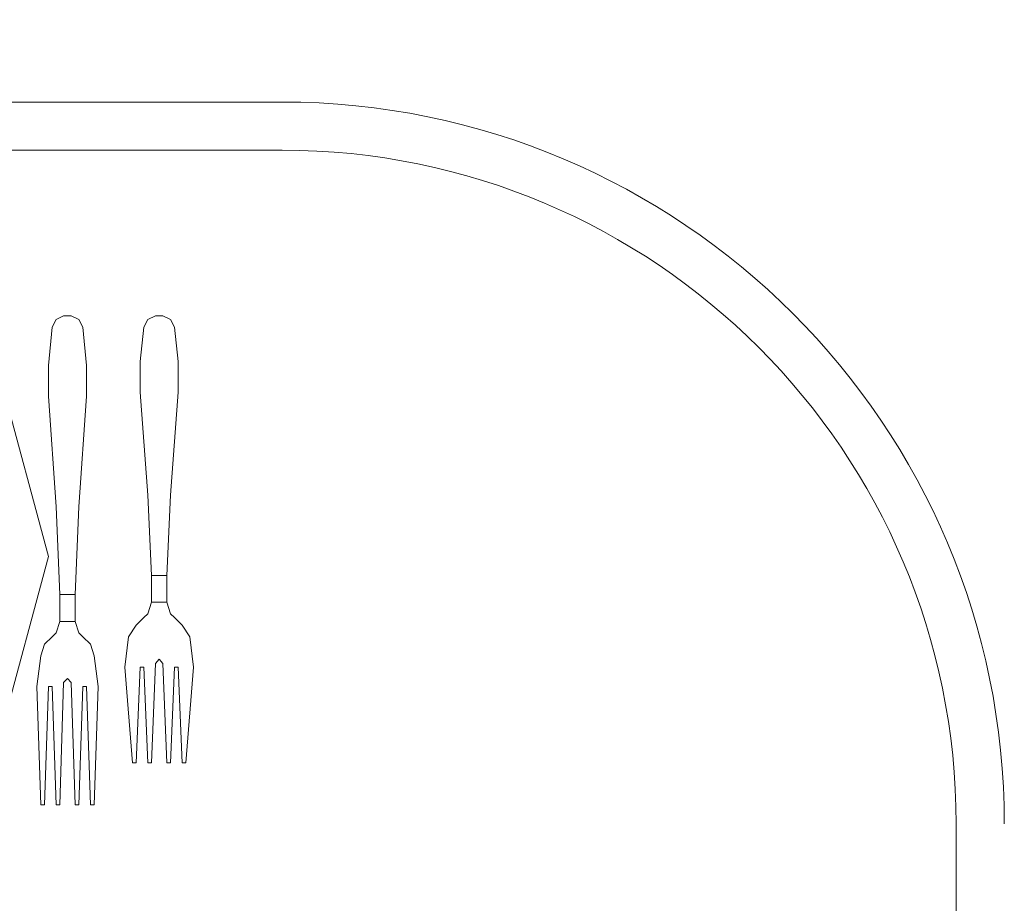
# Model space of a CAD drawing. Units: inches. Extents: x 375 to 1122, y 27 to 1069.
# Tile 64 of 155: x 731.16 to 747.02, y 311.59 to 325.82. Entities that reach past the tile are written whole.
import ezdxf

# ---------------------------------------------------------------- set-up
doc = ezdxf.new("R2010")
doc.units = ezdxf.units.IN
doc.layers.add('A-ANNO-DIMS', color=2, linetype='Continuous', lineweight=18)
doc.layers.add('Furniture', color=30, linetype='Continuous', lineweight=18)
doc.styles.get("Standard").update_dxf_attribs({"font": 'arial.ttf'})
doc.dimstyles.new('ISO-25', dxfattribs={"dimtxt": 12, "dimasz": 2.5, "dimexe": 1.5, "dimexo": 1.5, "dimtad": 1, "dimdec": 1, "dimlunit": 3, "dimtxsty": 'Standard', "dimblk": 'ARCHTICK', "dimcen": 2.5, "dimadec": 0, "dimazin": 0, "dimtfac": 1, "dimtdec": 1, "dimtmove": 0, "dimatfit": 3, "dimfxl": 1.5, "dimfxlon": 1, "dimarcsym": 0})

# ---------------------------------------------------------------- blocks, each defined once
blk = doc.blocks.new('A$C403C54AD')
for p, q in [((0.83575, 1.53256, -0.0006), (1.99923, 1.53256, -0.0006)), ((0.54488, 0.79569, -0.0006), (0.54488, 1.26108, -0.0006)), ((0.56427, 0.79569, -0.0006), (0.56427, 1.26108, -0.0006)), ((0.76029, 1.22386, -0.03201), (0.75567, 1.22078, -0.03155)), ((0.76029, 1.22386, -0.03509), (0.75567, 1.22078, -0.03463)), ((0.76798, 1.18538, -0.03201), (0.76336, 1.18384, -0.03155)), ((0.76798, 1.18538, -0.03509), (0.76336, 1.18384, -0.03463))]:
    blk.add_line(p, q)
for radius in [0.29087, 0.27148]:
    blk.add_arc((0.83575, 1.26108, -0.0006), radius, 90, 180)
for points, invisible_edges in [([(0.75567, 1.20231, -0.03155), (0.75567, 1.22078, -0.03155), (0.76029, 1.22386, -0.03201), (0.76029, 1.19923, -0.03201)], 5), ([(0.75567, 1.20231, -0.03463), (0.75567, 1.22078, -0.03463), (0.76029, 1.22386, -0.03509), (0.76029, 1.19923, -0.03509)], 5), ([(0.75567, 1.22078, -0.03155), (0.75567, 1.22078, -0.03463), (0.76029, 1.22386, -0.03509), (0.76029, 1.22386, -0.03201)], 4), ([(0.76029, 1.22386, -0.03201), (0.7726, 1.2177, -0.03141), (0.7726, 1.21924, -0.03141), (0.7726, 1.2254, -0.03141)], 5), ([(0.76029, 1.22386, -0.03509), (0.7726, 1.2177, -0.03449), (0.7726, 1.21924, -0.03449), (0.7726, 1.2254, -0.03449)], 5), ([(0.76029, 1.22386, -0.03509), (0.76029, 1.22386, -0.03201), (0.7726, 1.2254, -0.03141), (0.7726, 1.2254, -0.03449)], 1), ([(0.76029, 1.22386, -0.03201), (0.7694, 1.21155, -0.0318), (0.77106, 1.21308, -0.03166), (0.7726, 1.2177, -0.03141)], 13), ([(0.76029, 1.19923, -0.03201), (0.7694, 1.21155, -0.0318), (0.76029, 1.22386, -0.03201), (0.76029, 1.19923, -0.03201)], 7), ([(0.76029, 1.22386, -0.03509), (0.7694, 1.21155, -0.03488), (0.77106, 1.21308, -0.03473), (0.7726, 1.2177, -0.03449)], 13), ([(0.76029, 1.19923, -0.03509), (0.7694, 1.21155, -0.03488), (0.76029, 1.22386, -0.03509), (0.76029, 1.19923, -0.03509)], 7), ([(0.7726, 1.21924, -0.03141), (0.7726, 1.2254, -0.03141), (0.81108, 1.22232, -0.02431), (0.81108, 1.22078, -0.02431)], 1), ([(0.7726, 1.21924, -0.03449), (0.7726, 1.2254, -0.03449), (0.81108, 1.22232, -0.02739), (0.81108, 1.22078, -0.02739)], 1), ([(0.63253, 1.20693, -0.03017), (0.63253, 1.21616, -0.03017), (0.63561, 1.2177, -0.03041), (0.63561, 1.20539, -0.03041)], 5), ([(0.63253, 1.20693, -0.03481), (0.63253, 1.21616, -0.03481), (0.63561, 1.2177, -0.03505), (0.63561, 1.20539, -0.03505)], 5), ([(0.63561, 1.2177, -0.03041), (0.63561, 1.20539, -0.03041), (0.64946, 1.20385, -0.03045), (0.64946, 1.21924, -0.03045)], 5), ([(0.63561, 1.2177, -0.03505), (0.63561, 1.20539, -0.03505), (0.64946, 1.20385, -0.03508), (0.64946, 1.21924, -0.03508)], 5), ([(0.64946, 1.20385, -0.03045), (0.64946, 1.21924, -0.03045), (0.66178, 1.21924, -0.03012), (0.66178, 1.20385, -0.03012)], 5), ([(0.64946, 1.20385, -0.03508), (0.64946, 1.21924, -0.03508), (0.66178, 1.21924, -0.03476), (0.66178, 1.20385, -0.03476)], 5), ([(0.66178, 1.21924, -0.03012), (0.66178, 1.20385, -0.03012), (0.70334, 1.20693, -0.02774), (0.70334, 1.21616, -0.02774)], 5), ([(0.66178, 1.21924, -0.03476), (0.66178, 1.20385, -0.03476), (0.70334, 1.20693, -0.03082), (0.70334, 1.21616, -0.03082)], 5), ([(0.70334, 1.21616, -0.03082), (0.70334, 1.21616, -0.02774), (0.66178, 1.21924, -0.03012), (0.66178, 1.21924, -0.03476)], 1), ([(0.75105, 1.21616, -0.02926), (0.75105, 1.20693, -0.02926), (0.75259, 1.20539, -0.03031), (0.75259, 1.2177, -0.03031)], 5), ([(0.75105, 1.21616, -0.03205), (0.75105, 1.20693, -0.03205), (0.75259, 1.20539, -0.03339), (0.75259, 1.2177, -0.03339)], 5), ([(0.75105, 1.21616, -0.02926), (0.75105, 1.21616, -0.03205), (0.75259, 1.2177, -0.03339), (0.75259, 1.2177, -0.03031)], 1), ([(0.75259, 1.2177, -0.03339), (0.75259, 1.20539, -0.03339), (0.75567, 1.20231, -0.03463), (0.75567, 1.22078, -0.03463)], 5), ([(0.75259, 1.2177, -0.03031), (0.75259, 1.20539, -0.03031), (0.75567, 1.20231, -0.03155), (0.75567, 1.22078, -0.03155)], 5), ([(0.77106, 1.21308, -0.03166), (0.7726, 1.2177, -0.03141), (0.81108, 1.21616, -0.02431), (0.81108, 1.21462, -0.02431)], 1), ([(0.77106, 1.21308, -0.03473), (0.7726, 1.2177, -0.03449), (0.81108, 1.21616, -0.02739), (0.81108, 1.21462, -0.02739)], 1), ([(0.63099, 1.21308, -0.03034), (0.63099, 1.21001, -0.03034), (0.63253, 1.20693, -0.03017), (0.63253, 1.21616, -0.03017)], 4), ([(0.63099, 1.21308, -0.03447), (0.63099, 1.21001, -0.03447), (0.63253, 1.20693, -0.03481), (0.63253, 1.21616, -0.03481)], 4), ([(0.70334, 1.20693, -0.02774), (0.70334, 1.21616, -0.02774), (0.73566, 1.21462, -0.02483), (0.73566, 1.20847, -0.02483)], 1), ([(0.73566, 1.21462, -0.02483), (0.73566, 1.21462, -0.02742), (0.70334, 1.21616, -0.03082), (0.70334, 1.21616, -0.02774)], 5), ([(0.70334, 1.20693, -0.03082), (0.70334, 1.21616, -0.03082), (0.73566, 1.21462, -0.02742), (0.73566, 1.20847, -0.02742)], 1), ([(0.74643, 1.21462, -0.0295), (0.74643, 1.21462, -0.02691), (0.73566, 1.21462, -0.02483), (0.73566, 1.21462, -0.02742)], 5), ([(0.74643, 1.20847, -0.02691), (0.74643, 1.21462, -0.02691), (0.75105, 1.21616, -0.02926), (0.75105, 1.20693, -0.02926)], 4), ([(0.74643, 1.20847, -0.0295), (0.74643, 1.21462, -0.0295), (0.75105, 1.21616, -0.03205), (0.75105, 1.20693, -0.03205)], 4), ([(0.74643, 1.21462, -0.0295), (0.74643, 1.21462, -0.02691), (0.75105, 1.21616, -0.02926), (0.75105, 1.21616, -0.03205)], 5), ([(0.76029, 1.19923, -0.03201), (0.7694, 1.21155, -0.0318), (0.77106, 1.21001, -0.03166), (0.7726, 1.20539, -0.03141)], 13), ([(0.76029, 1.19923, -0.03509), (0.7694, 1.21155, -0.03488), (0.77106, 1.21001, -0.03473), (0.7726, 1.20539, -0.03449)], 13), ([(0.7726, 1.20539, -0.03141), (0.77106, 1.21001, -0.03166), (0.81108, 1.20847, -0.02431), (0.81108, 1.20693, -0.02431)], 1), ([(0.7726, 1.20539, -0.03449), (0.77106, 1.21001, -0.03473), (0.81108, 1.20847, -0.02739), (0.81108, 1.20693, -0.02739)], 1), ([(0.66178, 1.20385, -0.03476), (0.66178, 1.20385, -0.03012), (0.70334, 1.20693, -0.02774), (0.70334, 1.20693, -0.03082)], 4), ([(0.70334, 1.20693, -0.02774), (0.70334, 1.20693, -0.03082), (0.73566, 1.20847, -0.02742), (0.73566, 1.20847, -0.02483)], 5), ([(0.73566, 1.20847, -0.02742), (0.73566, 1.20847, -0.02483), (0.74643, 1.20847, -0.02691), (0.74643, 1.20847, -0.0295)], 5), ([(0.74643, 1.20847, -0.02691), (0.74643, 1.20847, -0.0295), (0.75105, 1.20693, -0.03205), (0.75105, 1.20693, -0.02926)], 5), ([(0.75105, 1.20693, -0.03205), (0.75105, 1.20693, -0.02926), (0.75259, 1.20539, -0.03031), (0.75259, 1.20539, -0.03339)], 1), ([(0.75567, 1.20231, -0.03463), (0.75567, 1.20231, -0.03155), (0.76029, 1.19923, -0.03201), (0.76029, 1.19923, -0.03509)], 4), ([(0.76029, 1.19923, -0.03201), (0.7726, 1.20539, -0.03141), (0.7726, 1.20385, -0.03141), (0.7726, 1.19769, -0.03141)], 5), ([(0.76029, 1.19923, -0.03509), (0.7726, 1.20539, -0.03449), (0.7726, 1.20385, -0.03449), (0.7726, 1.19769, -0.03449)], 5), ([(0.7726, 1.20385, -0.03141), (0.7726, 1.19769, -0.03141), (0.81108, 1.20077, -0.02431), (0.81108, 1.20231, -0.02431)], 1), ([(0.7726, 1.20385, -0.03449), (0.7726, 1.19769, -0.03449), (0.81108, 1.20077, -0.02739), (0.81108, 1.20231, -0.02739)], 1), ([(0.76029, 1.19923, -0.03201), (0.76029, 1.19923, -0.03509), (0.7726, 1.19769, -0.03449), (0.7726, 1.19769, -0.03141)], 1), ([(0.76798, 1.18538, -0.03201), (0.7803, 1.18076, -0.03141), (0.7803, 1.1823, -0.03141), (0.7803, 1.18692, -0.03141)], 5), ([(0.76798, 1.18538, -0.03509), (0.7803, 1.18076, -0.03449), (0.7803, 1.1823, -0.03449), (0.7803, 1.18692, -0.03449)], 5), ([(0.76798, 1.18538, -0.03509), (0.76798, 1.18538, -0.03201), (0.7803, 1.18692, -0.03141), (0.7803, 1.18692, -0.03449)], 1), ([(0.7803, 1.1823, -0.03141), (0.7803, 1.18692, -0.03141), (0.82801, 1.18538, -0.02431), (0.82801, 1.18384, -0.02431)], 1), ([(0.7803, 1.1823, -0.03449), (0.7803, 1.18692, -0.03449), (0.82801, 1.18538, -0.02739), (0.82801, 1.18384, -0.02739)], 1), ([(0.63561, 1.18076, -0.03041), (0.63561, 1.16845, -0.03041), (0.651, 1.16691, -0.03045), (0.651, 1.1823, -0.03045)], 5), ([(0.63561, 1.18076, -0.03505), (0.63561, 1.16845, -0.03505), (0.651, 1.16691, -0.03508), (0.651, 1.1823, -0.03508)], 5), ([(0.651, 1.16691, -0.03045), (0.651, 1.1823, -0.03045), (0.66332, 1.1823, -0.03012), (0.66332, 1.16691, -0.03012)], 5), ([(0.651, 1.16691, -0.03508), (0.651, 1.1823, -0.03508), (0.66332, 1.1823, -0.03476), (0.66332, 1.16691, -0.03476)], 5), ([(0.66332, 1.1823, -0.03012), (0.66332, 1.16691, -0.03012), (0.70795, 1.16999, -0.02774), (0.70795, 1.17922, -0.02774)], 5), ([(0.66332, 1.1823, -0.03476), (0.66332, 1.16691, -0.03476), (0.70795, 1.16999, -0.03082), (0.70795, 1.17922, -0.03082)], 5), ([(0.70795, 1.17922, -0.03082), (0.70795, 1.17922, -0.02774), (0.66332, 1.1823, -0.03012), (0.66332, 1.1823, -0.03476)], 1), ([(0.76029, 1.18076, -0.03339), (0.76029, 1.16845, -0.03339), (0.76336, 1.16537, -0.03463), (0.76336, 1.18384, -0.03463)], 5), ([(0.76029, 1.18076, -0.03031), (0.76029, 1.16845, -0.03031), (0.76336, 1.16537, -0.03155), (0.76336, 1.18384, -0.03155)], 5), ([(0.76336, 1.16537, -0.03155), (0.76336, 1.18384, -0.03155), (0.76798, 1.18538, -0.03201), (0.76798, 1.16383, -0.03201)], 5), ([(0.76336, 1.16537, -0.03463), (0.76336, 1.18384, -0.03463), (0.76798, 1.18538, -0.03509), (0.76798, 1.16383, -0.03509)], 5), ([(0.76336, 1.18384, -0.03155), (0.76336, 1.18384, -0.03463), (0.76798, 1.18538, -0.03509), (0.76798, 1.18538, -0.03201)], 4), ([(0.76798, 1.18538, -0.03201), (0.77709, 1.17461, -0.0318), (0.77876, 1.17614, -0.03166), (0.7803, 1.18076, -0.03141)], 13), ([(0.76798, 1.16383, -0.03201), (0.77709, 1.17461, -0.0318), (0.76798, 1.18538, -0.03201), (0.76798, 1.16383, -0.03201)], 7), ([(0.76798, 1.16383, -0.03509), (0.77709, 1.17461, -0.03488), (0.76798, 1.18538, -0.03509), (0.76798, 1.16383, -0.03509)], 7), ([(0.76798, 1.18538, -0.03509), (0.77709, 1.17461, -0.03488), (0.77876, 1.17614, -0.03473), (0.7803, 1.18076, -0.03449)], 13), ([(0.63099, 1.17614, -0.03034), (0.63099, 1.17307, -0.03034), (0.63253, 1.16999, -0.03017), (0.63253, 1.17922, -0.03017)], 4), ([(0.63099, 1.17614, -0.03447), (0.63099, 1.17307, -0.03447), (0.63253, 1.16999, -0.03481), (0.63253, 1.17922, -0.03481)], 4), ([(0.63253, 1.16999, -0.03017), (0.63253, 1.17922, -0.03017), (0.63561, 1.18076, -0.03041), (0.63561, 1.16845, -0.03041)], 5), ([(0.63253, 1.16999, -0.03481), (0.63253, 1.17922, -0.03481), (0.63561, 1.18076, -0.03505), (0.63561, 1.16845, -0.03505)], 5), ([(0.70795, 1.16999, -0.02774), (0.70795, 1.17922, -0.02774), (0.74335, 1.17768, -0.02483), (0.74335, 1.17153, -0.02483)], 1), ([(0.74335, 1.17768, -0.02483), (0.74335, 1.17768, -0.02742), (0.70795, 1.17922, -0.03082), (0.70795, 1.17922, -0.02774)], 5), ([(0.70795, 1.16999, -0.03082), (0.70795, 1.17922, -0.03082), (0.74335, 1.17768, -0.02742), (0.74335, 1.17153, -0.02742)], 1), ([(0.75413, 1.17153, -0.02691), (0.75413, 1.17768, -0.02691), (0.75875, 1.17922, -0.02926), (0.75875, 1.16999, -0.02926)], 4), ([(0.75413, 1.17768, -0.0295), (0.75413, 1.17768, -0.02691), (0.75875, 1.17922, -0.02926), (0.75875, 1.17922, -0.03205)], 5), ([(0.75413, 1.17153, -0.0295), (0.75413, 1.17768, -0.0295), (0.75875, 1.17922, -0.03205), (0.75875, 1.16999, -0.03205)], 4), ([(0.75875, 1.17922, -0.02926), (0.75875, 1.16999, -0.02926), (0.76029, 1.16845, -0.03031), (0.76029, 1.18076, -0.03031)], 5), ([(0.75875, 1.17922, -0.03205), (0.75875, 1.16999, -0.03205), (0.76029, 1.16845, -0.03339), (0.76029, 1.18076, -0.03339)], 5), ([(0.75875, 1.17922, -0.02926), (0.75875, 1.17922, -0.03205), (0.76029, 1.18076, -0.03339), (0.76029, 1.18076, -0.03031)], 1), ([(0.77876, 1.17614, -0.03166), (0.7803, 1.18076, -0.03141), (0.82801, 1.17922, -0.02431), (0.82801, 1.17768, -0.02431)], 1), ([(0.77876, 1.17614, -0.03473), (0.7803, 1.18076, -0.03449), (0.82801, 1.17922, -0.02739), (0.82801, 1.17768, -0.02739)], 1), ([(0.75413, 1.17768, -0.0295), (0.75413, 1.17768, -0.02691), (0.74335, 1.17768, -0.02483), (0.74335, 1.17768, -0.02742)], 5), ([(0.76798, 1.16383, -0.03201), (0.77709, 1.17461, -0.0318), (0.77876, 1.17307, -0.03166), (0.7803, 1.16845, -0.03141)], 13), ([(0.76798, 1.16383, -0.03509), (0.77709, 1.17461, -0.03488), (0.77876, 1.17307, -0.03473), (0.7803, 1.16845, -0.03449)], 13), ([(0.66332, 1.16691, -0.03476), (0.66332, 1.16691, -0.03012), (0.70795, 1.16999, -0.02774), (0.70795, 1.16999, -0.03082)], 4), ([(0.70795, 1.16999, -0.02774), (0.70795, 1.16999, -0.03082), (0.74335, 1.17153, -0.02742), (0.74335, 1.17153, -0.02483)], 5), ([(0.74335, 1.17153, -0.02742), (0.74335, 1.17153, -0.02483), (0.75413, 1.17153, -0.02691), (0.75413, 1.17153, -0.0295)], 5), ([(0.75413, 1.17153, -0.02691), (0.75413, 1.17153, -0.0295), (0.75875, 1.16999, -0.03205), (0.75875, 1.16999, -0.02926)], 5), ([(0.75875, 1.16999, -0.03205), (0.75875, 1.16999, -0.02926), (0.76029, 1.16845, -0.03031), (0.76029, 1.16845, -0.03339)], 1), ([(0.7803, 1.16845, -0.03141), (0.77876, 1.17307, -0.03166), (0.82801, 1.17153, -0.02431), (0.82801, 1.16999, -0.02431)], 1), ([(0.7803, 1.16845, -0.03449), (0.77876, 1.17307, -0.03473), (0.82801, 1.17153, -0.02739), (0.82801, 1.16999, -0.02739)], 1), ([(0.76798, 1.16383, -0.03201), (0.7803, 1.16845, -0.03141), (0.7803, 1.16691, -0.03141), (0.7803, 1.16229, -0.03141)], 5), ([(0.76798, 1.16383, -0.03509), (0.7803, 1.16845, -0.03449), (0.7803, 1.16691, -0.03449), (0.7803, 1.16229, -0.03449)], 5), ([(0.7803, 1.16691, -0.03141), (0.7803, 1.16229, -0.03141), (0.82801, 1.16383, -0.02431), (0.82801, 1.16537, -0.02431)], 1), ([(0.7803, 1.16691, -0.03449), (0.7803, 1.16229, -0.03449), (0.82801, 1.16383, -0.02739), (0.82801, 1.16537, -0.02739)], 1), ([(0.76336, 1.16537, -0.03463), (0.76336, 1.16537, -0.03155), (0.76798, 1.16383, -0.03201), (0.76798, 1.16383, -0.03509)], 4), ([(0.76798, 1.16383, -0.03201), (0.76798, 1.16383, -0.03509), (0.7803, 1.16229, -0.03449), (0.7803, 1.16229, -0.03141)], 1)]:
    blk.add_3dface(points, dxfattribs=dict(invisible_edges=invisible_edges))
for points in [[(0.81108, 1.22232, -0.02431), (0.81108, 1.22232, -0.02739), (0.7726, 1.2254, -0.03449), (0.7726, 1.2254, -0.03141)], [(0.81108, 1.22078, -0.02739), (0.81108, 1.22078, -0.02431), (0.81108, 1.22232, -0.02431), (0.81108, 1.22232, -0.02739)], [(0.63561, 1.2177, -0.03041), (0.63561, 1.2177, -0.03505), (0.63253, 1.21616, -0.03481), (0.63253, 1.21616, -0.03017)], [(0.64946, 1.21924, -0.03508), (0.64946, 1.21924, -0.03045), (0.63561, 1.2177, -0.03041), (0.63561, 1.2177, -0.03505)], [(0.66178, 1.21924, -0.03012), (0.66178, 1.21924, -0.03476), (0.64946, 1.21924, -0.03508), (0.64946, 1.21924, -0.03045)], [(0.75259, 1.2177, -0.03339), (0.75259, 1.2177, -0.03031), (0.75567, 1.22078, -0.03155), (0.75567, 1.22078, -0.03463)], [(0.7726, 1.21924, -0.03141), (0.7726, 1.21924, -0.03449), (0.81108, 1.22078, -0.02739), (0.81108, 1.22078, -0.02431)], [(0.7726, 1.21924, -0.03141), (0.7726, 1.21924, -0.03449), (0.7726, 1.2177, -0.03449), (0.7726, 1.2177, -0.03141)], [(0.81108, 1.21616, -0.02431), (0.81108, 1.21616, -0.02739), (0.7726, 1.2177, -0.03449), (0.7726, 1.2177, -0.03141)], [(0.63253, 1.21616, -0.03481), (0.63253, 1.21616, -0.03017), (0.63099, 1.21308, -0.03034), (0.63099, 1.21308, -0.03447)], [(0.73566, 1.21462, -0.02483), (0.73566, 1.20847, -0.02483), (0.74643, 1.20847, -0.02691), (0.74643, 1.21462, -0.02691)], [(0.73566, 1.21462, -0.02742), (0.73566, 1.20847, -0.02742), (0.74643, 1.20847, -0.0295), (0.74643, 1.21462, -0.0295)], [(0.77106, 1.21308, -0.03473), (0.77106, 1.21308, -0.03166), (0.81108, 1.21462, -0.02431), (0.81108, 1.21462, -0.02739)], [(0.81108, 1.21462, -0.02739), (0.81108, 1.21462, -0.02431), (0.81108, 1.21616, -0.02431), (0.81108, 1.21616, -0.02739)], [(0.63099, 1.21308, -0.03034), (0.63099, 1.21308, -0.03447), (0.63099, 1.21001, -0.03447), (0.63099, 1.21001, -0.03034)], [(0.63099, 1.21001, -0.03447), (0.63099, 1.21001, -0.03034), (0.63253, 1.20693, -0.03017), (0.63253, 1.20693, -0.03481)], [(0.77106, 1.21308, -0.03166), (0.77106, 1.21308, -0.03473), (0.7694, 1.21155, -0.03488), (0.7694, 1.21155, -0.0318)], [(0.7694, 1.21155, -0.03488), (0.7694, 1.21155, -0.0318), (0.77106, 1.21001, -0.03166), (0.77106, 1.21001, -0.03473)], [(0.81108, 1.20847, -0.02739), (0.81108, 1.20847, -0.02431), (0.77106, 1.21001, -0.03166), (0.77106, 1.21001, -0.03473)], [(0.63253, 1.20693, -0.03017), (0.63253, 1.20693, -0.03481), (0.63561, 1.20539, -0.03505), (0.63561, 1.20539, -0.03041)], [(0.7726, 1.20539, -0.03449), (0.7726, 1.20539, -0.03141), (0.81108, 1.20693, -0.02431), (0.81108, 1.20693, -0.02739)], [(0.81108, 1.20693, -0.02739), (0.81108, 1.20693, -0.02431), (0.81108, 1.20847, -0.02431), (0.81108, 1.20847, -0.02739)], [(0.63561, 1.20539, -0.03505), (0.63561, 1.20539, -0.03041), (0.64946, 1.20385, -0.03045), (0.64946, 1.20385, -0.03508)], [(0.64946, 1.20385, -0.03045), (0.64946, 1.20385, -0.03508), (0.66178, 1.20385, -0.03476), (0.66178, 1.20385, -0.03012)], [(0.75259, 1.20539, -0.03031), (0.75259, 1.20539, -0.03339), (0.75567, 1.20231, -0.03463), (0.75567, 1.20231, -0.03155)], [(0.7726, 1.20539, -0.03449), (0.7726, 1.20539, -0.03141), (0.7726, 1.20385, -0.03141), (0.7726, 1.20385, -0.03449)], [(0.81108, 1.20231, -0.02431), (0.81108, 1.20231, -0.02739), (0.7726, 1.20385, -0.03449), (0.7726, 1.20385, -0.03141)], [(0.81108, 1.20077, -0.02739), (0.81108, 1.20077, -0.02431), (0.81108, 1.20231, -0.02431), (0.81108, 1.20231, -0.02739)], [(0.7726, 1.19769, -0.03449), (0.7726, 1.19769, -0.03141), (0.81108, 1.20077, -0.02431), (0.81108, 1.20077, -0.02739)], [(0.82801, 1.18538, -0.02431), (0.82801, 1.18538, -0.02739), (0.7803, 1.18692, -0.03449), (0.7803, 1.18692, -0.03141)], [(0.651, 1.1823, -0.03508), (0.651, 1.1823, -0.03045), (0.63561, 1.18076, -0.03041), (0.63561, 1.18076, -0.03505)], [(0.66332, 1.1823, -0.03012), (0.66332, 1.1823, -0.03476), (0.651, 1.1823, -0.03508), (0.651, 1.1823, -0.03045)], [(0.76029, 1.18076, -0.03339), (0.76029, 1.18076, -0.03031), (0.76336, 1.18384, -0.03155), (0.76336, 1.18384, -0.03463)], [(0.7803, 1.1823, -0.03141), (0.7803, 1.1823, -0.03449), (0.82801, 1.18384, -0.02739), (0.82801, 1.18384, -0.02431)], [(0.7803, 1.1823, -0.03141), (0.7803, 1.1823, -0.03449), (0.7803, 1.18076, -0.03449), (0.7803, 1.18076, -0.03141)], [(0.82801, 1.18384, -0.02739), (0.82801, 1.18384, -0.02431), (0.82801, 1.18538, -0.02431), (0.82801, 1.18538, -0.02739)], [(0.63253, 1.17922, -0.03481), (0.63253, 1.17922, -0.03017), (0.63099, 1.17614, -0.03034), (0.63099, 1.17614, -0.03447)], [(0.63561, 1.18076, -0.03041), (0.63561, 1.18076, -0.03505), (0.63253, 1.17922, -0.03481), (0.63253, 1.17922, -0.03017)], [(0.82801, 1.17922, -0.02431), (0.82801, 1.17922, -0.02739), (0.7803, 1.18076, -0.03449), (0.7803, 1.18076, -0.03141)], [(0.82801, 1.17768, -0.02739), (0.82801, 1.17768, -0.02431), (0.82801, 1.17922, -0.02431), (0.82801, 1.17922, -0.02739)], [(0.63099, 1.17614, -0.03034), (0.63099, 1.17614, -0.03447), (0.63099, 1.17307, -0.03447), (0.63099, 1.17307, -0.03034)], [(0.74335, 1.17768, -0.02483), (0.74335, 1.17153, -0.02483), (0.75413, 1.17153, -0.02691), (0.75413, 1.17768, -0.02691)], [(0.74335, 1.17768, -0.02742), (0.74335, 1.17153, -0.02742), (0.75413, 1.17153, -0.0295), (0.75413, 1.17768, -0.0295)], [(0.77876, 1.17614, -0.03166), (0.77876, 1.17614, -0.03473), (0.77709, 1.17461, -0.03488), (0.77709, 1.17461, -0.0318)], [(0.77709, 1.17461, -0.03488), (0.77709, 1.17461, -0.0318), (0.77876, 1.17307, -0.03166), (0.77876, 1.17307, -0.03473)], [(0.77876, 1.17614, -0.03473), (0.77876, 1.17614, -0.03166), (0.82801, 1.17768, -0.02431), (0.82801, 1.17768, -0.02739)], [(0.63099, 1.17307, -0.03447), (0.63099, 1.17307, -0.03034), (0.63253, 1.16999, -0.03017), (0.63253, 1.16999, -0.03481)], [(0.63253, 1.16999, -0.03017), (0.63253, 1.16999, -0.03481), (0.63561, 1.16845, -0.03505), (0.63561, 1.16845, -0.03041)], [(0.82801, 1.17153, -0.02739), (0.82801, 1.17153, -0.02431), (0.77876, 1.17307, -0.03166), (0.77876, 1.17307, -0.03473)], [(0.7803, 1.16845, -0.03449), (0.7803, 1.16845, -0.03141), (0.82801, 1.16999, -0.02431), (0.82801, 1.16999, -0.02739)], [(0.82801, 1.16999, -0.02739), (0.82801, 1.16999, -0.02431), (0.82801, 1.17153, -0.02431), (0.82801, 1.17153, -0.02739)], [(0.63561, 1.16845, -0.03505), (0.63561, 1.16845, -0.03041), (0.651, 1.16691, -0.03045), (0.651, 1.16691, -0.03508)], [(0.651, 1.16691, -0.03045), (0.651, 1.16691, -0.03508), (0.66332, 1.16691, -0.03476), (0.66332, 1.16691, -0.03012)], [(0.76029, 1.16845, -0.03031), (0.76029, 1.16845, -0.03339), (0.76336, 1.16537, -0.03463), (0.76336, 1.16537, -0.03155)], [(0.7803, 1.16845, -0.03449), (0.7803, 1.16845, -0.03141), (0.7803, 1.16691, -0.03141), (0.7803, 1.16691, -0.03449)], [(0.82801, 1.16537, -0.02431), (0.82801, 1.16537, -0.02739), (0.7803, 1.16691, -0.03449), (0.7803, 1.16691, -0.03141)], [(0.7803, 1.16229, -0.03449), (0.7803, 1.16229, -0.03141), (0.82801, 1.16383, -0.02431), (0.82801, 1.16383, -0.02739)], [(0.82801, 1.16383, -0.02739), (0.82801, 1.16383, -0.02431), (0.82801, 1.16537, -0.02431), (0.82801, 1.16537, -0.02739)]]:
    blk.add_3dface(points)
at = {"linetype": 'ByBlock', "invisible_edges": 5}
for points in [[(0.72796, 1.16691, -0.0197), (0.72796, 1.14844, -0.0197), (0.66793, 1.13235, -0.0197), (0.6587, 1.14835, -0.0197)], [(0.72796, 1.13305, -0.03355), (0.72796, 1.16691, -0.02431), (0.6587, 1.14835, -0.02431), (0.67563, 1.11902, -0.03355)], [(0.79723, 1.14835, -0.0197), (0.78799, 1.13235, -0.0197), (0.72796, 1.14844, -0.0197), (0.72796, 1.16691, -0.0197)], [(0.7803, 1.11902, -0.03355), (0.79723, 1.14835, -0.02431), (0.72796, 1.16691, -0.02431), (0.72796, 1.13305, -0.03355)]]:
    blk.add_3dface(points, dxfattribs=at)
at = {"linetype": 'ByBlock'}
for points in [[(0.72796, 1.16691, -0.02431), (0.72796, 1.16691, -0.0197), (0.6587, 1.14835, -0.0197), (0.6587, 1.14835, -0.02431)], [(0.79723, 1.14835, -0.02431), (0.79723, 1.14835, -0.0197), (0.72796, 1.16691, -0.0197), (0.72796, 1.16691, -0.02431)]]:
    blk.add_3dface(points, dxfattribs=at)
blk = doc.blocks.new('_ArchTick')
at = {"color": 0, "linetype": 'ByBlock', "const_width": 0.15}
blk.add_lwpolyline([(-0.5, -0.5), (0.5, 0.5)], dxfattribs=at)
blk = doc.blocks.new('*D94')
at = {"layer": 'A-ANNO-DIMS', "color": 0, "lineweight": -2, "transparency": 16777216}
for p, q in [((734.007, 117.528), (734.007, 114.528)), ((773.007, 117.528), (773.007, 114.528)), ((734.007, 116.028), (773.007, 116.028))]:
    blk.add_line(p, q, dxfattribs=at)
at = {"layer": 'Defpoints', "color": 0, "transparency": 16777216}
for p in [(734.007, 667.528), (773.007, 667.528), (773.007, 116.028)]:
    blk.add_point(p, dxfattribs=at)
at = {"layer": 'A-ANNO-DIMS', "color": 0, "lineweight": -2, "transparency": 16777216, "xscale": 2.5, "yscale": 2.5, "zscale": 2.5, "rotation": 180}
blk.add_blockref('_ArchTick', (734.007, 116.028), dxfattribs=at)
at = {"layer": 'A-ANNO-DIMS', "color": 0, "lineweight": -2, "transparency": 16777216, "xscale": 2.5, "yscale": 2.5, "zscale": 2.5}
blk.add_blockref('_ArchTick', (773.007, 116.028), dxfattribs=at)
at = {"layer": 'A-ANNO-DIMS', "color": 0, "transparency": 16777216, "insert": (753.507, 122.784), "char_height": 12, "attachment_point": 5}
blk.add_mtext('3\'-3"', dxfattribs=at)

msp = doc.modelspace()

# ---------------------------------------------------------------- block references
at = {"layer": 'Furniture', "xscale": 39.9918517141215, "yscale": 39.9918517141215, "zscale": 39.9918517141215, "rotation": 270}
msp.add_blockref('A$C403C54AD', (684.955, 346.287, 0.024), dxfattribs=at)

# ---------------------------------------------------------------- dimensions: what is measured, and where the dimension line sits
at = {"layer": 'A-ANNO-DIMS'}
dim = msp.add_linear_dim(base=(773.007, 116.028), p1=(734.007, 667.528), p2=(773.007, 667.528), dimstyle='ISO-25', override={"dimdec": 1, "dimlfac": 1, "dimrnd": 0, "dimzin": 1, "dimdsep": 46, "dimlunit": 4, "dimfrac": 2}, dxfattribs=at)
dim.commit()
dim.dimension.update_dxf_attribs({"geometry": '*D94', "text_midpoint": (753.507, 122.784)})

doc.saveas('drawing.dxf')
